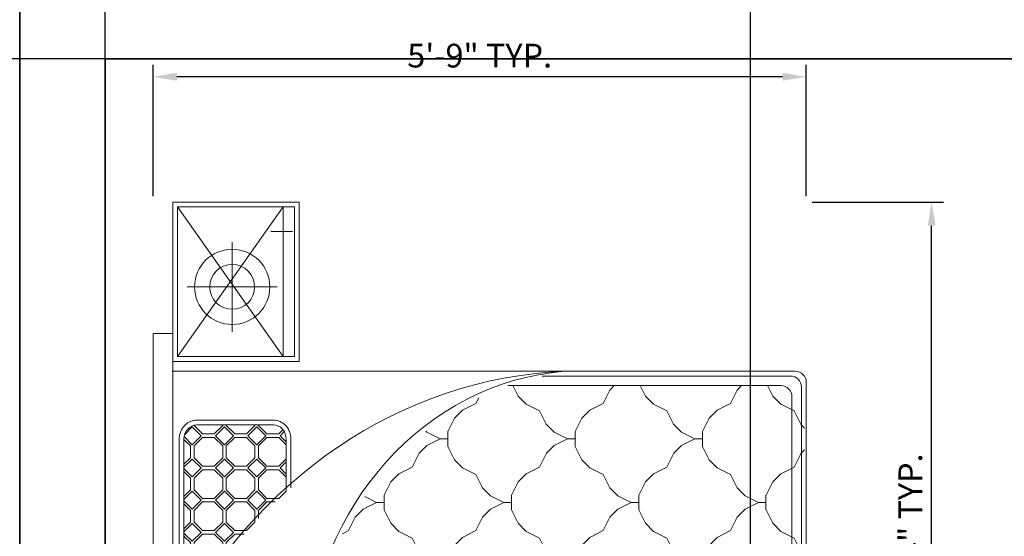
# Model space of a CAD drawing. Units: inches. Extents: x 1624 to 3956, y 1589 to 5028.
# Tile 13 of 16: x 1943 to 2046, y 2372 to 2426. Entities that reach past the tile are written whole.
import ezdxf

# ---------------------------------------------------------------- set-up
doc = ezdxf.new("R2010")
doc.units = ezdxf.units.IN
for name, color, linetype, lineweight in [('A-ANNO-DIMS', 2, 'Continuous', 13), ('A-FURN', 8, 'Continuous', 18), ('A-WALL', 7, 'Continuous', 35)]:
    doc.layers.add(name, color=color, linetype=linetype, lineweight=lineweight)
doc.styles.get("Standard").update_dxf_attribs({"font": 'arial.ttf'})
doc.dimstyles.new('Copy of ISO-25', dxfattribs={"dimtxt": 2.5, "dimasz": 2.5, "dimexe": 1.25, "dimexo": 0.625, "dimtad": 1, "dimdec": 1, "dimlunit": 4, "dimtxsty": 'Standard', "dimcen": 2.5, "dimadec": 0, "dimazin": 0, "dimtfac": 1, "dimtdec": 1, "dimtmove": 0, "dimatfit": 3, "dimfxl": 1, "dimarcsym": 0})

# ---------------------------------------------------------------- blocks, each defined once
blk = doc.blocks.new('A$C029D5C69')
for p, q in [((0.4164, 2.0693), (0.4164, 2.0066)), ((2.2315, 2.0693), (0.4164, 2.0693)), ((2.2315, 2.0066), (2.2315, 2.0693)), ((0, 1.606), (0, 2.0066)), ((0, 2.0066), (0.505, 2.0066)), ((0.4164, 2.0066), (2.2315, 2.0066)), ((0.505, 2.0066), (0.505, 1.606)), ((0.5252, 0.0351), (0.5252, 2.0066)), ((0.5403, 0.0502), (0.5403, 2.0066)), ((0.5706, 0.0805), (0.5706, 2.0066)), ((0.6869, 1.966), (0.6666, 2.0066)), ((0.7072, 2.0066), (0.6869, 1.966)), ((1.0902, 1.966), (1.0699, 2.0066)), ((1.1106, 2.0066), (1.0902, 1.966)), ((2.1114, 2.0087), (2.1114, 0.0351)), ((2.6479, 2.0066), (2.1429, 2.0066)), ((2.1429, 2.0066), (2.1429, 1.606)), ((2.6479, 1.606), (2.6479, 2.0066)), ((0.0151, 1.6211), (0.0151, 1.9915)), ((0.0151, 1.9915), (0.4899, 1.9915)), ((0.4899, 1.9915), (0.4899, 1.6211)), ((0.6869, 1.9425), (0.6869, 1.966)), ((0.6869, 1.9425), (0.6869, 1.966)), ((1.0902, 1.9425), (1.0902, 1.966)), ((1.0902, 1.9425), (1.0902, 1.966)), ((1.8954, 1.9865), (1.3081, 1.9865)), ((1.8954, 1.9713), (1.3339, 1.9713)), ((1.3849, 1.9713), (1.3656, 1.952)), ((1.3945, 1.9713), (1.3714, 1.9483)), ((1.4249, 1.945), (1.3986, 1.9713)), ((1.4288, 1.9507), (1.4081, 1.9713)), ((1.487, 1.9713), (1.4664, 1.9507)), ((1.4966, 1.9713), (1.4703, 1.945)), ((1.527, 1.945), (1.5007, 1.9713)), ((1.5309, 1.9507), (1.5102, 1.9713)), ((1.5891, 1.9713), (1.5685, 1.9507)), ((1.5987, 1.9713), (1.5724, 1.945)), ((1.6291, 1.945), (1.6028, 1.9713)), ((1.633, 1.9507), (1.6123, 1.9713)), ((1.6912, 1.9713), (1.6706, 1.9507)), ((1.7008, 1.9713), (1.6745, 1.945)), ((1.7312, 1.945), (1.7049, 1.9713)), ((1.7351, 1.9507), (1.7144, 1.9713)), ((1.7933, 1.9713), (1.7727, 1.9507)), ((1.8029, 1.9713), (1.7766, 1.945)), ((1.8333, 1.945), (1.807, 1.9713)), ((1.8372, 1.9507), (1.8165, 1.9713)), ((1.8954, 1.9713), (1.8748, 1.9507)), ((1.9043, 1.9707), (1.8787, 1.945)), ((1.9354, 1.945), (1.9114, 1.969)), ((2.6328, 1.9915), (2.158, 1.9915)), ((2.158, 1.9915), (2.158, 1.6211)), ((2.6328, 1.6211), (2.6328, 1.9915)), ((0.2689, 1.9609), (0.2689, 1.6764)), ((0.6634, 1.9425), (0.621, 1.9213)), ((0.6634, 1.9425), (0.621, 1.9213)), ((0.6869, 1.9425), (0.6634, 1.9425)), ((0.6869, 1.9425), (0.7104, 1.9425)), ((0.7528, 1.9213), (0.7104, 1.9425)), ((0.7528, 1.9213), (0.7104, 1.9425)), ((1.0668, 1.9425), (1.0244, 1.9213)), ((1.0668, 1.9425), (1.0244, 1.9213)), ((1.0902, 1.9425), (1.0668, 1.9425)), ((1.0902, 1.9425), (1.1137, 1.9425)), ((1.1561, 1.9213), (1.1137, 1.9425)), ((1.1561, 1.9213), (1.1137, 1.9425)), ((1.4249, 1.945), (1.4059, 1.926)), ((1.4288, 1.9394), (1.4116, 1.9222)), ((1.4476, 1.9507), (1.4288, 1.9507)), ((1.4288, 1.9393), (1.4476, 1.9393)), ((1.4476, 1.9507), (1.4664, 1.9507)), ((1.4664, 1.9393), (1.4476, 1.9393)), ((1.493, 1.9128), (1.4664, 1.9394)), ((1.4986, 1.9167), (1.4703, 1.945)), ((1.527, 1.945), (1.4986, 1.9167)), ((1.5309, 1.9394), (1.5043, 1.9128)), ((1.5497, 1.9507), (1.5309, 1.9507)), ((1.5309, 1.9393), (1.5497, 1.9393)), ((1.5497, 1.9507), (1.5685, 1.9507)), ((1.5685, 1.9393), (1.5497, 1.9393)), ((1.595, 1.9128), (1.5685, 1.9394)), ((1.6007, 1.9167), (1.5724, 1.945)), ((1.6291, 1.945), (1.6007, 1.9167)), ((1.633, 1.9394), (1.6064, 1.9128)), ((1.6518, 1.9507), (1.633, 1.9507)), ((1.633, 1.9393), (1.6518, 1.9393)), ((1.6518, 1.9507), (1.6706, 1.9507)), ((1.6706, 1.9393), (1.6518, 1.9393)), ((1.6971, 1.9128), (1.6706, 1.9394)), ((1.7028, 1.9167), (1.6745, 1.945)), ((1.7312, 1.945), (1.7028, 1.9167)), ((1.7351, 1.9394), (1.7085, 1.9128)), ((1.7539, 1.9507), (1.7351, 1.9507)), ((1.7351, 1.9393), (1.7539, 1.9393)), ((1.7539, 1.9507), (1.7727, 1.9507)), ((1.7727, 1.9393), (1.7539, 1.9393)), ((1.7992, 1.9128), (1.7727, 1.9394)), ((1.8049, 1.9167), (1.7766, 1.945)), ((1.8333, 1.945), (1.8049, 1.9167)), ((1.8372, 1.9394), (1.8106, 1.9128)), ((1.856, 1.9507), (1.8372, 1.9507)), ((1.8372, 1.9393), (1.856, 1.9393)), ((1.856, 1.9507), (1.8748, 1.9507)), ((1.8748, 1.9393), (1.856, 1.9393)), ((1.9013, 1.9128), (1.8748, 1.9394)), ((1.907, 1.9167), (1.8787, 1.945)), ((1.9354, 1.945), (1.907, 1.9167)), ((1.9393, 1.9394), (1.9127, 1.9128)), ((1.9393, 1.9393), (1.9404, 1.9393)), ((2.379, 1.9609), (2.379, 1.6764)), ((0.621, 1.9213), (0.5955, 1.8958)), ((0.7783, 1.8958), (0.7528, 1.9213)), ((1.0243, 1.9213), (0.9988, 1.8958)), ((1.1816, 1.8958), (1.1561, 1.9213)), ((1.493, 1.8752), (1.493, 1.9128)), ((1.5043, 1.8752), (1.5043, 1.9128)), ((1.595, 1.8752), (1.595, 1.9128)), ((1.6064, 1.8752), (1.6064, 1.9128)), ((1.6971, 1.8752), (1.6971, 1.9128)), ((1.7085, 1.8752), (1.7085, 1.9128)), ((1.7992, 1.8752), (1.7992, 1.9128)), ((1.8106, 1.8752), (1.8106, 1.9128)), ((1.9013, 1.8752), (1.9013, 1.9128)), ((1.9127, 1.8752), (1.9127, 1.9128)), ((1.9414, 1.688), (1.9414, 1.931)), ((1.9565, 1.688), (1.9565, 1.931)), ((0.5955, 1.8958), (0.5743, 1.8534)), ((0.7995, 1.8534), (0.7783, 1.8958)), ((0.9989, 1.8958), (0.9777, 1.8534)), ((1.2028, 1.8534), (1.1816, 1.8958)), ((1.493, 1.8752), (1.4867, 1.869)), ((1.5309, 1.8486), (1.5043, 1.8752)), ((1.595, 1.8752), (1.5685, 1.8486)), ((1.633, 1.8486), (1.6064, 1.8752)), ((1.6971, 1.8752), (1.6706, 1.8486)), ((1.7351, 1.8486), (1.7085, 1.8752)), ((1.7992, 1.8752), (1.7727, 1.8486)), ((1.8372, 1.8486), (1.8106, 1.8752)), ((1.9013, 1.8752), (1.8748, 1.8486)), ((1.9393, 1.8486), (1.9127, 1.8752)), ((0.5743, 1.8534), (0.5706, 1.8515)), ((0.5743, 1.8534), (0.5706, 1.8515)), ((0.8419, 1.8322), (0.7995, 1.8534)), ((0.8419, 1.8322), (0.7995, 1.8534)), ((0.9777, 1.8534), (0.9353, 1.8322)), ((0.9777, 1.8534), (0.9353, 1.8322)), ((1.2452, 1.8322), (1.2028, 1.8534)), ((1.2452, 1.8322), (1.2028, 1.8534)), ((1.4986, 1.8713), (1.4922, 1.8648)), ((1.527, 1.8429), (1.4986, 1.8713)), ((1.527, 1.8429), (1.5242, 1.8401)), ((1.5497, 1.8486), (1.5309, 1.8486)), ((1.5497, 1.8486), (1.5685, 1.8486)), ((1.6007, 1.8713), (1.5724, 1.8429)), ((1.6007, 1.8146), (1.5724, 1.8429)), ((1.6291, 1.8429), (1.6007, 1.8713)), ((1.6291, 1.8429), (1.6007, 1.8146)), ((1.6518, 1.8486), (1.633, 1.8486)), ((1.6518, 1.8486), (1.6706, 1.8486)), ((1.7028, 1.8713), (1.6745, 1.8429)), ((1.7028, 1.8146), (1.6745, 1.8429)), ((1.7312, 1.8429), (1.7028, 1.8713)), ((1.7312, 1.8429), (1.7028, 1.8146)), ((1.7539, 1.8486), (1.7351, 1.8486)), ((1.7539, 1.8486), (1.7727, 1.8486)), ((1.8049, 1.8713), (1.7766, 1.8429)), ((1.8049, 1.8146), (1.7766, 1.8429)), ((1.8333, 1.8429), (1.8049, 1.8713)), ((1.8333, 1.8429), (1.8049, 1.8146)), ((1.856, 1.8486), (1.8372, 1.8486)), ((1.856, 1.8486), (1.8748, 1.8486)), ((1.907, 1.8713), (1.8787, 1.8429)), ((1.907, 1.8146), (1.8787, 1.8429)), ((1.9354, 1.8429), (1.907, 1.8713)), ((1.9354, 1.8429), (1.907, 1.8146)), ((1.9414, 1.8486), (1.9393, 1.8486)), ((0.1267, 1.8186), (0.4111, 1.8186)), ((0.8674, 1.8067), (0.8419, 1.8322)), ((0.9352, 1.8322), (0.9097, 1.8067)), ((1.2707, 1.8067), (1.2452, 1.8322)), ((1.5309, 1.8373), (1.5295, 1.8359)), ((1.5309, 1.8373), (1.5497, 1.8373)), ((1.5685, 1.8373), (1.5497, 1.8373)), ((1.595, 1.8107), (1.5685, 1.8373)), ((1.595, 1.7806), (1.595, 1.8107)), ((1.633, 1.8373), (1.6064, 1.8107)), ((1.6064, 1.7731), (1.6064, 1.8107)), ((1.633, 1.8373), (1.6518, 1.8373)), ((1.6706, 1.8373), (1.6518, 1.8373)), ((1.6971, 1.8107), (1.6706, 1.8373)), ((1.6971, 1.7731), (1.6971, 1.8107)), ((1.7351, 1.8373), (1.7085, 1.8107)), ((1.7085, 1.7731), (1.7085, 1.8107)), ((1.7351, 1.8373), (1.7539, 1.8373)), ((1.7727, 1.8373), (1.7539, 1.8373)), ((1.7992, 1.8107), (1.7727, 1.8373)), ((1.7992, 1.7731), (1.7992, 1.8107)), ((1.8372, 1.8373), (1.8106, 1.8107)), ((1.8106, 1.7731), (1.8106, 1.8107)), ((1.8372, 1.8373), (1.856, 1.8373)), ((1.8748, 1.8373), (1.856, 1.8373)), ((1.9013, 1.8107), (1.8748, 1.8373)), ((1.9013, 1.7731), (1.9013, 1.8107)), ((1.9393, 1.8373), (1.9127, 1.8107)), ((1.9127, 1.7731), (1.9127, 1.8107)), ((1.9393, 1.8373), (1.9414, 1.8373)), ((2.2367, 1.8186), (2.5212, 1.8186)), ((0.8886, 1.7643), (0.8674, 1.8067)), ((0.9098, 1.8067), (0.8886, 1.7643)), ((1.2919, 1.7643), (1.2707, 1.8067)), ((0.8886, 1.7408), (0.8886, 1.7643)), ((1.2981, 1.7768), (1.2919, 1.7643)), ((1.2919, 1.7519), (1.2919, 1.7643)), ((1.633, 1.7465), (1.6064, 1.7731)), ((1.6971, 1.7731), (1.6706, 1.7465)), ((1.7028, 1.7692), (1.6745, 1.7408)), ((1.7312, 1.7408), (1.7028, 1.7692)), ((1.7351, 1.7465), (1.7085, 1.7731)), ((1.7992, 1.7731), (1.7727, 1.7465)), ((1.8049, 1.7692), (1.7766, 1.7408)), ((1.8333, 1.7408), (1.8049, 1.7692)), ((1.8372, 1.7465), (1.8106, 1.7731)), ((1.9013, 1.7731), (1.8748, 1.7465)), ((1.907, 1.7692), (1.8787, 1.7408)), ((1.9354, 1.7408), (1.907, 1.7692)), ((1.9393, 1.7465), (1.9127, 1.7731)), ((0.8227, 1.7196), (0.7972, 1.6941)), ((0.8651, 1.7408), (0.8227, 1.7196)), ((0.8651, 1.7408), (0.8227, 1.7196)), ((0.912, 1.7408), (0.8651, 1.7408)), ((0.9544, 1.7196), (0.912, 1.7408)), ((0.9544, 1.7196), (0.912, 1.7408)), ((0.98, 1.6941), (0.9545, 1.7196)), ((1.226, 1.7196), (1.2005, 1.6941)), ((1.2684, 1.7408), (1.226, 1.7196)), ((1.2684, 1.7408), (1.226, 1.7196)), ((1.2885, 1.7408), (1.2684, 1.7408)), ((1.6518, 1.7465), (1.633, 1.7465)), ((1.6443, 1.7352), (1.6518, 1.7352)), ((1.6518, 1.7465), (1.6706, 1.7465)), ((1.6706, 1.7352), (1.6518, 1.7352)), ((1.6971, 1.7086), (1.6706, 1.7352)), ((1.7028, 1.7125), (1.6745, 1.7408)), ((1.7312, 1.7408), (1.7028, 1.7125)), ((1.7351, 1.7352), (1.7085, 1.7086)), ((1.7539, 1.7465), (1.7351, 1.7465)), ((1.7351, 1.7352), (1.7539, 1.7352)), ((1.7539, 1.7465), (1.7727, 1.7465)), ((1.7727, 1.7352), (1.7539, 1.7352)), ((1.7992, 1.7086), (1.7727, 1.7352)), ((1.8049, 1.7125), (1.7766, 1.7408)), ((1.8333, 1.7408), (1.8049, 1.7125)), ((1.8372, 1.7352), (1.8106, 1.7086)), ((1.856, 1.7465), (1.8372, 1.7465)), ((1.8372, 1.7352), (1.856, 1.7352)), ((1.856, 1.7465), (1.8748, 1.7465)), ((1.8748, 1.7352), (1.856, 1.7352)), ((1.9013, 1.7086), (1.8748, 1.7352)), ((1.907, 1.7125), (1.8787, 1.7408)), ((1.9354, 1.7408), (1.907, 1.7125)), ((1.9393, 1.7352), (1.9127, 1.7086)), ((1.9414, 1.7465), (1.9393, 1.7465)), ((1.9393, 1.7352), (1.9414, 1.7352)), ((0.5766, 1.6941), (0.5706, 1.7002)), ((0.5978, 1.6517), (0.5766, 1.6941)), ((0.7972, 1.6941), (0.776, 1.6517)), ((1.0011, 1.6517), (0.9799, 1.6941)), ((1.2005, 1.6941), (1.1793, 1.6517)), ((1.6971, 1.682), (1.6971, 1.7086)), ((1.7085, 1.671), (1.7085, 1.7086)), ((1.7992, 1.671), (1.7992, 1.7086)), ((1.8106, 1.671), (1.8106, 1.7086)), ((1.9013, 1.671), (1.9013, 1.7086)), ((1.9127, 1.671), (1.9127, 1.7086)), ((2.5551, 1.6275), (2.5551, 1.696)), ((1.7318, 1.6477), (1.7085, 1.671)), ((1.7992, 1.671), (1.7759, 1.6477)), ((1.8049, 1.6671), (1.7855, 1.6477)), ((1.8244, 1.6477), (1.8049, 1.6671)), ((1.8339, 1.6477), (1.8106, 1.671)), ((1.9013, 1.671), (1.878, 1.6477)), ((1.907, 1.6671), (1.8876, 1.6477)), ((1.9202, 1.6539), (1.907, 1.6671)), ((1.926, 1.6577), (1.9127, 1.671)), ((0.6402, 1.6305), (0.5978, 1.6517)), ((0.6402, 1.6305), (0.5978, 1.6517)), ((0.6657, 1.605), (0.6402, 1.6305)), ((0.7336, 1.6305), (0.7081, 1.605)), ((0.776, 1.6517), (0.7336, 1.6305)), ((0.776, 1.6517), (0.7336, 1.6305)), ((1.0435, 1.6305), (1.0011, 1.6517)), ((1.0435, 1.6305), (1.0011, 1.6517)), ((1.0691, 1.605), (1.0436, 1.6305)), ((1.1369, 1.6305), (1.1114, 1.605)), ((1.1793, 1.6517), (1.1369, 1.6305)), ((1.1793, 1.6517), (1.1369, 1.6305)), ((1.8961, 1.6477), (1.7289, 1.6477)), ((1.8961, 1.6325), (1.7422, 1.6325)), ((0.505, 1.606), (0, 1.606)), ((0.4899, 1.6211), (0.0151, 1.6211)), ((0.6869, 1.5626), (0.6657, 1.605)), ((0.7081, 1.605), (0.6869, 1.5626)), ((1.0902, 1.5626), (1.069, 1.605)), ((1.1114, 1.605), (1.0902, 1.5626)), ((2.1429, 1.606), (2.6479, 1.606)), ((2.158, 1.6211), (2.6328, 1.6211)), ((0.6869, 1.5392), (0.6869, 1.5626)), ((0.6869, 1.5392), (0.6869, 1.5626)), ((1.0902, 1.5392), (1.0902, 1.5626)), ((1.0902, 1.5392), (1.0902, 1.5626)), ((0.6634, 1.5391), (0.621, 1.5179)), ((0.6634, 1.5391), (0.621, 1.5179)), ((0.6869, 1.5392), (0.6634, 1.5392)), ((0.6869, 1.5392), (0.7104, 1.5392)), ((0.7528, 1.5179), (0.7104, 1.5391)), ((0.7528, 1.5179), (0.7104, 1.5391)), ((1.0668, 1.5391), (1.0244, 1.5179)), ((1.0668, 1.5391), (1.0244, 1.5179)), ((1.0902, 1.5392), (1.0668, 1.5392)), ((1.0902, 1.5392), (1.1137, 1.5392)), ((1.1561, 1.5179), (1.1137, 1.5391)), ((1.1561, 1.5179), (1.1137, 1.5391)), ((1.4534, 1.5308), (1.4277, 1.5179)), ((1.4534, 1.5308), (1.4277, 1.5179)), ((0.621, 1.5179), (0.5955, 1.4924)), ((0.7783, 1.4924), (0.7528, 1.5179)), ((1.0243, 1.5179), (0.9988, 1.4924)), ((1.1816, 1.4924), (1.1561, 1.5179)), ((1.4277, 1.5179), (1.4022, 1.4924)), ((0.5955, 1.4925), (0.5743, 1.4501)), ((0.7995, 1.4501), (0.7783, 1.4925)), ((0.9989, 1.4925), (0.9777, 1.4501)), ((1.2028, 1.4501), (1.1816, 1.4925)), ((1.4022, 1.4925), (1.381, 1.4501)), ((1.6062, 1.4501), (1.5966, 1.4692)), ((0.5743, 1.45), (0.5706, 1.4481)), ((0.5743, 1.45), (0.5706, 1.4481)), ((0.8419, 1.4288), (0.7995, 1.45)), ((0.8419, 1.4288), (0.7995, 1.45)), ((0.9777, 1.45), (0.9353, 1.4288)), ((0.9777, 1.45), (0.9353, 1.4288)), ((1.2452, 1.4288), (1.2028, 1.45)), ((1.2452, 1.4288), (1.2028, 1.45)), ((1.381, 1.45), (1.3386, 1.4288)), ((1.381, 1.45), (1.3386, 1.4288)), ((1.6486, 1.4288), (1.6062, 1.45)), ((1.6486, 1.4288), (1.6062, 1.45)), ((0.5403, 1.4117), (0.5706, 1.4117)), ((0.8674, 1.4033), (0.8419, 1.4288)), ((0.9352, 1.4288), (0.9097, 1.4033)), ((1.2707, 1.4033), (1.2452, 1.4288)), ((1.3386, 1.4288), (1.3131, 1.4033)), ((1.6741, 1.4033), (1.6486, 1.4288)), ((0.8886, 1.361), (0.8674, 1.4034)), ((0.9098, 1.4034), (0.8886, 1.361)), ((1.2919, 1.361), (1.2707, 1.4034)), ((1.3131, 1.4034), (1.2919, 1.361)), ((1.6953, 1.361), (1.6741, 1.4034)), ((1.714, 1.3984), (1.6953, 1.361)), ((0.8886, 1.3375), (0.8886, 1.3609)), ((1.2919, 1.3375), (1.2919, 1.3609)), ((1.6953, 1.3375), (1.6953, 1.3609)), ((0.8227, 1.3163), (0.7972, 1.2908)), ((0.8651, 1.3374), (0.8227, 1.3162)), ((0.8651, 1.3374), (0.8227, 1.3162)), ((0.912, 1.3375), (0.8651, 1.3375)), ((0.9544, 1.3162), (0.912, 1.3374)), ((0.9544, 1.3162), (0.912, 1.3374)), ((0.98, 1.2908), (0.9545, 1.3163)), ((1.226, 1.3163), (1.2005, 1.2908)), ((1.2684, 1.3374), (1.226, 1.3162)), ((1.2684, 1.3374), (1.226, 1.3162)), ((1.3154, 1.3375), (1.2684, 1.3375)), ((1.3578, 1.3162), (1.3154, 1.3374)), ((1.3578, 1.3162), (1.3154, 1.3374)), ((1.3833, 1.2908), (1.3578, 1.3163)), ((1.6294, 1.3163), (1.6039, 1.2908)), ((1.6718, 1.3374), (1.6294, 1.3162)), ((1.6718, 1.3374), (1.6294, 1.3162)), ((1.7187, 1.3375), (1.6718, 1.3375)), ((1.7611, 1.3162), (1.7187, 1.3374)), ((1.7611, 1.3162), (1.7187, 1.3374)), ((1.7867, 1.2908), (1.7611, 1.3163)), ((0.5766, 1.2908), (0.5706, 1.2968)), ((0.5978, 1.2484), (0.5766, 1.2908)), ((0.7972, 1.2908), (0.776, 1.2484)), ((1.0011, 1.2484), (0.9799, 1.2908)), ((1.2005, 1.2908), (1.1793, 1.2484)), ((1.4045, 1.2484), (1.3833, 1.2908)), ((1.6039, 1.2908), (1.5827, 1.2484)), ((1.8078, 1.2484), (1.7866, 1.2908)), ((0.6402, 1.2271), (0.5978, 1.2483)), ((0.6402, 1.2271), (0.5978, 1.2483)), ((0.776, 1.2483), (0.7336, 1.2271)), ((0.776, 1.2483), (0.7336, 1.2271)), ((1.0435, 1.2271), (1.0011, 1.2483)), ((1.0435, 1.2271), (1.0011, 1.2483)), ((1.1793, 1.2483), (1.1369, 1.2271)), ((1.1793, 1.2483), (1.1369, 1.2271)), ((1.4469, 1.2271), (1.4045, 1.2483)), ((1.4469, 1.2271), (1.4045, 1.2483)), ((1.5827, 1.2483), (1.5403, 1.2271)), ((1.5827, 1.2483), (1.5403, 1.2271)), ((1.8502, 1.2271), (1.8078, 1.2483)), ((1.8502, 1.2271), (1.8078, 1.2483)), ((0.6657, 1.2017), (0.6402, 1.2272)), ((0.7336, 1.2272), (0.7081, 1.2017)), ((1.0691, 1.2017), (1.0436, 1.2272)), ((1.1369, 1.2272), (1.1114, 1.2017)), ((1.4724, 1.2017), (1.4469, 1.2272)), ((1.5403, 1.2272), (1.5148, 1.2017)), ((1.8758, 1.2017), (1.8503, 1.2272)), ((0.5403, 1.21), (0.5706, 1.21)), ((0.6869, 1.1593), (0.6657, 1.2017)), ((0.7081, 1.2017), (0.6869, 1.1593)), ((1.0902, 1.1593), (1.069, 1.2017)), ((1.1114, 1.2017), (1.0902, 1.1593)), ((1.4936, 1.1593), (1.4724, 1.2017)), ((1.5148, 1.2017), (1.4936, 1.1593)), ((1.8969, 1.1593), (1.8757, 1.2017)), ((1.9181, 1.2017), (1.8969, 1.1593)), ((1.9215, 1.2051), (1.9181, 1.2017)), ((0.6869, 1.1358), (0.6869, 1.1593)), ((0.6869, 1.1358), (0.6869, 1.1593)), ((1.0902, 1.1358), (1.0902, 1.1593)), ((1.0902, 1.1358), (1.0902, 1.1593)), ((1.4936, 1.1358), (1.4936, 1.1593)), ((1.4936, 1.1358), (1.4936, 1.1593)), ((1.8969, 1.1358), (1.8969, 1.1593)), ((1.8969, 1.1358), (1.8969, 1.1593)), ((0.6634, 1.1358), (0.621, 1.1146)), ((0.6634, 1.1358), (0.621, 1.1146)), ((0.6869, 1.1358), (0.6634, 1.1358)), ((0.6869, 1.1358), (0.7104, 1.1358)), ((0.7528, 1.1146), (0.7104, 1.1358)), ((0.7528, 1.1146), (0.7104, 1.1358)), ((1.0668, 1.1358), (1.0244, 1.1146)), ((1.0668, 1.1358), (1.0244, 1.1146)), ((1.0902, 1.1358), (1.0668, 1.1358)), ((1.0902, 1.1358), (1.1137, 1.1358)), ((1.1561, 1.1146), (1.1137, 1.1358)), ((1.1561, 1.1146), (1.1137, 1.1358)), ((1.4701, 1.1358), (1.4277, 1.1146)), ((1.4701, 1.1358), (1.4277, 1.1146)), ((1.4936, 1.1358), (1.4701, 1.1358)), ((1.4936, 1.1358), (1.5171, 1.1358)), ((1.5595, 1.1146), (1.5171, 1.1358)), ((1.5595, 1.1146), (1.5171, 1.1358)), ((1.8735, 1.1358), (1.8311, 1.1146)), ((1.8735, 1.1358), (1.8311, 1.1146)), ((1.8969, 1.1358), (1.8735, 1.1358)), ((1.8969, 1.1358), (1.9204, 1.1358)), ((1.9628, 1.1146), (1.9204, 1.1358)), ((1.9628, 1.1146), (1.9204, 1.1358)), ((0.621, 1.1146), (0.5955, 1.0891)), ((0.7783, 1.0891), (0.7528, 1.1146)), ((1.0243, 1.1146), (0.9988, 1.0891)), ((1.1816, 1.0891), (1.1561, 1.1146)), ((1.4277, 1.1146), (1.4022, 1.0891)), ((1.585, 1.0891), (1.5595, 1.1146)), ((1.831, 1.1146), (1.8055, 1.0891)), ((1.9883, 1.0891), (1.9628, 1.1146)), ((0.5955, 1.0891), (0.5743, 1.0467)), ((0.7995, 1.0467), (0.7783, 1.0891)), ((0.9989, 1.0891), (0.9777, 1.0467)), ((1.2028, 1.0467), (1.1816, 1.0891)), ((1.4022, 1.0891), (1.381, 1.0467)), ((1.6062, 1.0467), (1.585, 1.0891)), ((1.8056, 1.0891), (1.7844, 1.0467)), ((2.0095, 1.0467), (1.9883, 1.0891)), ((0.5743, 1.0467), (0.5706, 1.0448)), ((0.5743, 1.0467), (0.5706, 1.0448)), ((0.8419, 1.0255), (0.7995, 1.0467)), ((0.8419, 1.0255), (0.7995, 1.0467)), ((0.9777, 1.0467), (0.9353, 1.0255)), ((0.9777, 1.0467), (0.9353, 1.0255)), ((1.2452, 1.0255), (1.2028, 1.0467)), ((1.2452, 1.0255), (1.2028, 1.0467)), ((1.381, 1.0467), (1.3386, 1.0255)), ((1.381, 1.0467), (1.3386, 1.0255)), ((1.6486, 1.0255), (1.6062, 1.0467)), ((1.6486, 1.0255), (1.6062, 1.0467)), ((1.7844, 1.0467), (1.742, 1.0255)), ((1.7844, 1.0467), (1.742, 1.0255)), ((2.0276, 1.0376), (2.0095, 1.0467)), ((2.0276, 1.0376), (2.0095, 1.0467)), ((0.8674, 1), (0.8419, 1.0255)), ((0.8886, 0.9576), (0.8674, 1)), ((0.9098, 1), (0.8886, 0.9576)), ((0.9352, 1.0255), (0.9097, 1)), ((1.2707, 1), (1.2452, 1.0255)), ((1.2919, 0.9576), (1.2707, 1)), ((1.3131, 1), (1.2919, 0.9576)), ((1.3386, 1.0255), (1.3131, 1)), ((1.6741, 1), (1.6486, 1.0255)), ((1.6953, 0.9576), (1.6741, 1)), ((1.7165, 1), (1.6953, 0.9576)), ((1.7419, 1.0255), (1.7164, 1)), ((0.8886, 0.9341), (0.8886, 0.9576)), ((1.2919, 0.9341), (1.2919, 0.9576)), ((1.6953, 0.9341), (1.6953, 0.9576)), ((2.066, 0.9457), (2.066, 0.0805)), ((0.8227, 0.9129), (0.7972, 0.8874)), ((0.8651, 0.9341), (0.8227, 0.9129)), ((0.8651, 0.9341), (0.8227, 0.9129)), ((0.912, 0.9341), (0.8651, 0.9341)), ((0.9544, 0.9129), (0.912, 0.9341)), ((0.9544, 0.9129), (0.912, 0.9341)), ((0.98, 0.8874), (0.9545, 0.9129)), ((1.226, 0.9129), (1.2005, 0.8874)), ((1.2684, 0.9341), (1.226, 0.9129)), ((1.2684, 0.9341), (1.226, 0.9129)), ((1.3154, 0.9341), (1.2684, 0.9341)), ((1.3578, 0.9129), (1.3154, 0.9341)), ((1.3578, 0.9129), (1.3154, 0.9341)), ((1.3833, 0.8874), (1.3578, 0.9129)), ((1.6294, 0.9129), (1.6039, 0.8874)), ((1.6718, 0.9341), (1.6294, 0.9129)), ((1.6718, 0.9341), (1.6294, 0.9129)), ((1.7187, 0.9341), (1.6718, 0.9341)), ((1.7611, 0.9129), (1.7187, 0.9341)), ((1.7611, 0.9129), (1.7187, 0.9341)), ((1.7867, 0.8874), (1.7611, 0.9129)), ((2.0327, 0.9129), (2.0072, 0.8874)), ((2.066, 0.9295), (2.0327, 0.9129)), ((2.066, 0.9295), (2.0327, 0.9129)), ((0.5766, 0.8874), (0.5706, 0.8935)), ((0.5978, 0.845), (0.5766, 0.8874)), ((0.7972, 0.8874), (0.776, 0.845)), ((1.0011, 0.845), (0.9799, 0.8874)), ((1.2005, 0.8874), (1.1793, 0.845)), ((1.4045, 0.845), (1.3833, 0.8874)), ((1.6039, 0.8874), (1.5827, 0.845)), ((1.8078, 0.845), (1.7866, 0.8874)), ((2.0072, 0.8874), (1.986, 0.845)), ((0.6402, 0.8238), (0.5978, 0.845)), ((0.6402, 0.8238), (0.5978, 0.845)), ((0.776, 0.845), (0.7336, 0.8238)), ((0.776, 0.845), (0.7336, 0.8238)), ((1.0435, 0.8238), (1.0011, 0.845)), ((1.0435, 0.8238), (1.0011, 0.845)), ((1.1793, 0.845), (1.1369, 0.8238)), ((1.1793, 0.845), (1.1369, 0.8238)), ((1.4469, 0.8238), (1.4045, 0.845)), ((1.4469, 0.8238), (1.4045, 0.845)), ((1.5827, 0.845), (1.5403, 0.8238)), ((1.5827, 0.845), (1.5403, 0.8238)), ((1.8502, 0.8238), (1.8078, 0.845)), ((1.8502, 0.8238), (1.8078, 0.845)), ((1.986, 0.845), (1.9436, 0.8238)), ((1.986, 0.845), (1.9436, 0.8238)), ((0.6657, 0.7983), (0.6402, 0.8238)), ((0.7336, 0.8238), (0.7081, 0.7983)), ((1.0691, 0.7983), (1.0436, 0.8238)), ((1.1369, 0.8238), (1.1114, 0.7983)), ((1.4724, 0.7983), (1.4469, 0.8238)), ((1.5403, 0.8238), (1.5148, 0.7983)), ((1.8758, 0.7983), (1.8503, 0.8238)), ((1.9436, 0.8238), (1.9181, 0.7983)), ((2.0962, 0.8369), (2.0962, 0.0502)), ((0.6869, 0.7559), (0.6657, 0.7983)), ((0.7081, 0.7983), (0.6869, 0.7559)), ((1.0902, 0.7559), (1.069, 0.7983)), ((1.1114, 0.7983), (1.0902, 0.7559)), ((1.4936, 0.7559), (1.4724, 0.7983)), ((1.5148, 0.7983), (1.4936, 0.7559)), ((1.8969, 0.7559), (1.8757, 0.7983)), ((1.9181, 0.7983), (1.8969, 0.7559)), ((0.6869, 0.7325), (0.6869, 0.7559)), ((0.6869, 0.7325), (0.6869, 0.7559)), ((1.0902, 0.7325), (1.0902, 0.7559)), ((1.0902, 0.7325), (1.0902, 0.7559)), ((1.2024, 0.7028), (1.2503, 0.7507)), ((1.4936, 0.7325), (1.4936, 0.7559)), ((1.4936, 0.7325), (1.4936, 0.7559)), ((1.8969, 0.7325), (1.8969, 0.7559)), ((1.8969, 0.7325), (1.8969, 0.7559)), ((0.6634, 0.7324), (0.621, 0.7112)), ((0.6634, 0.7324), (0.621, 0.7112)), ((0.6869, 0.7325), (0.6634, 0.7325)), ((0.6869, 0.7325), (0.7104, 0.7325)), ((0.7528, 0.7112), (0.7104, 0.7324)), ((0.7528, 0.7112), (0.7104, 0.7324)), ((1.0668, 0.7324), (1.0244, 0.7112)), ((1.0668, 0.7324), (1.0244, 0.7112)), ((1.0902, 0.7325), (1.0668, 0.7325)), ((1.0902, 0.7325), (1.1137, 0.7325)), ((1.1561, 0.7112), (1.1137, 0.7324)), ((1.1561, 0.7112), (1.1137, 0.7324)), ((1.4701, 0.7324), (1.4277, 0.7112)), ((1.4701, 0.7324), (1.4277, 0.7112)), ((1.4936, 0.7325), (1.4701, 0.7325)), ((1.4936, 0.7325), (1.5171, 0.7325)), ((1.5595, 0.7112), (1.5171, 0.7324)), ((1.5595, 0.7112), (1.5171, 0.7324)), ((1.8735, 0.7324), (1.8311, 0.7112)), ((1.8735, 0.7324), (1.8311, 0.7112)), ((1.8969, 0.7325), (1.8735, 0.7325)), ((1.8969, 0.7325), (1.9204, 0.7325)), ((1.9628, 0.7112), (1.9204, 0.7324)), ((1.9628, 0.7112), (1.9204, 0.7324)), ((0.621, 0.7113), (0.5955, 0.6858)), ((0.7783, 0.6858), (0.7528, 0.7113)), ((1.0243, 0.7113), (0.9988, 0.6858)), ((1.1816, 0.6858), (1.1561, 0.7113)), ((1.4277, 0.7113), (1.4022, 0.6858)), ((1.585, 0.6858), (1.5595, 0.7113)), ((1.831, 0.7113), (1.8055, 0.6858)), ((1.9883, 0.6858), (1.9628, 0.7113)), ((0.5955, 0.6858), (0.5743, 0.6434)), ((0.7995, 0.6434), (0.7783, 0.6858)), ((0.9989, 0.6858), (0.9777, 0.6434)), ((1.2028, 0.6434), (1.1816, 0.6858)), ((1.4022, 0.6858), (1.381, 0.6434)), ((1.6062, 0.6434), (1.585, 0.6858)), ((1.8056, 0.6858), (1.7844, 0.6434)), ((2.0095, 0.6434), (1.9883, 0.6858)), ((0.5743, 0.6433), (0.5706, 0.6414)), ((0.5743, 0.6433), (0.5706, 0.6414)), ((0.8419, 0.6221), (0.7995, 0.6433)), ((0.8419, 0.6221), (0.7995, 0.6433)), ((0.9777, 0.6433), (0.9353, 0.6221)), ((0.9777, 0.6433), (0.9353, 0.6221)), ((1.2452, 0.6221), (1.2028, 0.6433)), ((1.2452, 0.6221), (1.2028, 0.6433)), ((1.381, 0.6433), (1.3386, 0.6221)), ((1.381, 0.6433), (1.3386, 0.6221)), ((1.6486, 0.6221), (1.6062, 0.6433)), ((1.6486, 0.6221), (1.6062, 0.6433)), ((1.7844, 0.6433), (1.742, 0.6221)), ((1.7844, 0.6433), (1.742, 0.6221)), ((2.0519, 0.6221), (2.0095, 0.6433)), ((2.0519, 0.6221), (2.0095, 0.6433)), ((0.8674, 0.5967), (0.8419, 0.6222)), ((0.8886, 0.5543), (0.8674, 0.5967)), ((0.9098, 0.5967), (0.8886, 0.5543)), ((0.9352, 0.6222), (0.9097, 0.5967)), ((1.2707, 0.5967), (1.2452, 0.6222)), ((1.2919, 0.5543), (1.2707, 0.5967)), ((1.3131, 0.5967), (1.2919, 0.5543)), ((1.3386, 0.6222), (1.3131, 0.5967)), ((1.6741, 0.5967), (1.6486, 0.6222)), ((1.6953, 0.5543), (1.6741, 0.5967)), ((1.7165, 0.5967), (1.6953, 0.5543)), ((1.7419, 0.6222), (1.7164, 0.5967)), ((2.066, 0.6081), (2.0519, 0.6222)), ((0.8651, 0.5308), (0.8227, 0.5096)), ((0.8651, 0.5308), (0.8227, 0.5096)), ((0.912, 0.5308), (0.8651, 0.5308)), ((0.8886, 0.5308), (0.8886, 0.5543)), ((0.9544, 0.5096), (0.912, 0.5308)), ((0.9544, 0.5096), (0.912, 0.5308)), ((1.2684, 0.5308), (1.226, 0.5096)), ((1.2684, 0.5308), (1.226, 0.5096)), ((1.3154, 0.5308), (1.2684, 0.5308)), ((1.2919, 0.5308), (1.2919, 0.5543)), ((1.3578, 0.5096), (1.3154, 0.5308)), ((1.3578, 0.5096), (1.3154, 0.5308)), ((1.6718, 0.5308), (1.6294, 0.5096)), ((1.6718, 0.5308), (1.6294, 0.5096)), ((1.7187, 0.5308), (1.6718, 0.5308)), ((1.6953, 0.5308), (1.6953, 0.5543)), ((1.7611, 0.5096), (1.7187, 0.5308)), ((1.7611, 0.5096), (1.7187, 0.5308)), ((0.8227, 0.5096), (0.7972, 0.4841)), ((0.98, 0.4841), (0.9545, 0.5096)), ((1.226, 0.5096), (1.2005, 0.4841)), ((1.3833, 0.4841), (1.3578, 0.5096)), ((1.6294, 0.5096), (1.6039, 0.4841)), ((1.7867, 0.4841), (1.7611, 0.5096)), ((2.0327, 0.5096), (2.0072, 0.4841)), ((2.066, 0.5262), (2.0327, 0.5096)), ((2.066, 0.5262), (2.0327, 0.5096)), ((0.5766, 0.4841), (0.5706, 0.4901)), ((0.5978, 0.4417), (0.5766, 0.4841)), ((0.7972, 0.4841), (0.776, 0.4417)), ((1.0011, 0.4417), (0.9799, 0.4841)), ((1.2005, 0.4841), (1.1793, 0.4417)), ((1.4045, 0.4417), (1.3833, 0.4841)), ((1.6039, 0.4841), (1.5827, 0.4417)), ((1.8078, 0.4417), (1.7866, 0.4841)), ((2.0072, 0.4841), (1.986, 0.4417)), ((0.6402, 0.4205), (0.5978, 0.4417)), ((0.6402, 0.4205), (0.5978, 0.4417)), ((0.776, 0.4417), (0.7336, 0.4205)), ((0.776, 0.4417), (0.7336, 0.4205)), ((1.0435, 0.4205), (1.0011, 0.4417)), ((1.0435, 0.4205), (1.0011, 0.4417)), ((1.1793, 0.4417), (1.1369, 0.4205)), ((1.1793, 0.4417), (1.1369, 0.4205)), ((1.4469, 0.4205), (1.4045, 0.4417)), ((1.4469, 0.4205), (1.4045, 0.4417)), ((1.5827, 0.4417), (1.5403, 0.4205)), ((1.5827, 0.4417), (1.5403, 0.4205)), ((1.8502, 0.4205), (1.8078, 0.4417)), ((1.8502, 0.4205), (1.8078, 0.4417)), ((1.986, 0.4417), (1.9436, 0.4205)), ((1.986, 0.4417), (1.9436, 0.4205)), ((0.6657, 0.395), (0.6402, 0.4205)), ((0.7336, 0.4205), (0.7081, 0.395)), ((1.0691, 0.395), (1.0436, 0.4205)), ((1.1369, 0.4205), (1.1114, 0.395)), ((1.4724, 0.395), (1.4469, 0.4205)), ((1.5403, 0.4205), (1.5148, 0.395)), ((1.8758, 0.395), (1.8503, 0.4205)), ((1.9436, 0.4205), (1.9181, 0.395)), ((0.6869, 0.3526), (0.6657, 0.395)), ((0.7081, 0.395), (0.6869, 0.3526)), ((1.0902, 0.3526), (1.069, 0.395)), ((1.1114, 0.395), (1.0902, 0.3526)), ((1.4936, 0.3526), (1.4724, 0.395)), ((1.5148, 0.395), (1.4936, 0.3526)), ((1.8969, 0.3526), (1.8757, 0.395)), ((1.9181, 0.395), (1.8969, 0.3526)), ((0.6869, 0.3291), (0.6869, 0.3526)), ((0.6869, 0.3291), (0.6869, 0.3526)), ((1.0902, 0.3291), (1.0902, 0.3526)), ((1.0902, 0.3291), (1.0902, 0.3526)), ((1.4936, 0.3291), (1.4936, 0.3526)), ((1.4936, 0.3291), (1.4936, 0.3526)), ((1.8969, 0.3291), (1.8969, 0.3526)), ((1.8969, 0.3291), (1.8969, 0.3526)), ((0.6634, 0.3291), (0.621, 0.3079)), ((0.6634, 0.3291), (0.621, 0.3079)), ((0.6869, 0.3291), (0.6634, 0.3291)), ((0.6869, 0.3291), (0.7104, 0.3291)), ((0.7528, 0.3079), (0.7104, 0.3291)), ((0.7528, 0.3079), (0.7104, 0.3291)), ((1.0668, 0.3291), (1.0244, 0.3079)), ((1.0668, 0.3291), (1.0244, 0.3079)), ((1.0902, 0.3291), (1.0668, 0.3291)), ((1.0902, 0.3291), (1.1137, 0.3291)), ((1.1561, 0.3079), (1.1137, 0.3291)), ((1.1561, 0.3079), (1.1137, 0.3291)), ((1.4701, 0.3291), (1.4277, 0.3079)), ((1.4701, 0.3291), (1.4277, 0.3079)), ((1.4936, 0.3291), (1.4701, 0.3291)), ((1.4936, 0.3291), (1.5171, 0.3291)), ((1.5595, 0.3079), (1.5171, 0.3291)), ((1.5595, 0.3079), (1.5171, 0.3291)), ((1.8735, 0.3291), (1.8311, 0.3079)), ((1.8735, 0.3291), (1.8311, 0.3079)), ((1.8969, 0.3291), (1.8735, 0.3291)), ((1.8969, 0.3291), (1.9204, 0.3291)), ((1.9628, 0.3079), (1.9204, 0.3291)), ((1.9628, 0.3079), (1.9204, 0.3291)), ((0.5955, 0.2824), (0.5743, 0.24)), ((0.621, 0.3079), (0.5955, 0.2824)), ((0.7783, 0.2824), (0.7528, 0.3079)), ((0.7995, 0.24), (0.7783, 0.2824)), ((0.9989, 0.2824), (0.9777, 0.24)), ((1.0243, 0.3079), (0.9988, 0.2824)), ((1.1816, 0.2824), (1.1561, 0.3079)), ((1.2028, 0.24), (1.1816, 0.2824)), ((1.4022, 0.2824), (1.381, 0.24)), ((1.4277, 0.3079), (1.4022, 0.2824)), ((1.585, 0.2824), (1.5595, 0.3079)), ((1.6062, 0.24), (1.585, 0.2824)), ((1.8056, 0.2824), (1.7844, 0.24)), ((1.831, 0.3079), (1.8055, 0.2824)), ((1.9883, 0.2824), (1.9628, 0.3079)), ((2.0095, 0.24), (1.9883, 0.2824)), ((0.5743, 0.24), (0.5706, 0.2381)), ((0.5743, 0.24), (0.5706, 0.2381)), ((0.8419, 0.2188), (0.7995, 0.24)), ((0.8419, 0.2188), (0.7995, 0.24)), ((0.8674, 0.1933), (0.8419, 0.2188)), ((0.9352, 0.2188), (0.9097, 0.1933)), ((0.9777, 0.24), (0.9353, 0.2188)), ((0.9777, 0.24), (0.9353, 0.2188)), ((1.2452, 0.2188), (1.2028, 0.24)), ((1.2452, 0.2188), (1.2028, 0.24)), ((1.2707, 0.1933), (1.2452, 0.2188)), ((1.3386, 0.2188), (1.3131, 0.1933)), ((1.381, 0.24), (1.3386, 0.2188)), ((1.381, 0.24), (1.3386, 0.2188)), ((1.6486, 0.2188), (1.6062, 0.24)), ((1.6486, 0.2188), (1.6062, 0.24)), ((1.6741, 0.1933), (1.6486, 0.2188)), ((1.7419, 0.2188), (1.7164, 0.1933)), ((1.7844, 0.24), (1.742, 0.2188)), ((1.7844, 0.24), (1.742, 0.2188)), ((2.0519, 0.2188), (2.0095, 0.24)), ((2.0519, 0.2188), (2.0095, 0.24)), ((2.066, 0.2047), (2.0519, 0.2188)), ((0.8886, 0.1509), (0.8674, 0.1933)), ((0.9098, 0.1933), (0.8886, 0.1509)), ((1.2919, 0.1509), (1.2707, 0.1933)), ((1.3131, 0.1933), (1.2919, 0.1509)), ((1.6953, 0.1509), (1.6741, 0.1933)), ((1.7165, 0.1933), (1.6953, 0.1509)), ((0.8651, 0.1274), (0.8227, 0.1062)), ((0.8651, 0.1274), (0.8227, 0.1062)), ((0.912, 0.1275), (0.8651, 0.1275)), ((0.8886, 0.1275), (0.8886, 0.1509)), ((0.9544, 0.1062), (0.912, 0.1274)), ((0.9544, 0.1062), (0.912, 0.1274)), ((1.2684, 0.1274), (1.226, 0.1062)), ((1.2684, 0.1274), (1.226, 0.1062)), ((1.3154, 0.1275), (1.2684, 0.1275)), ((1.2919, 0.1275), (1.2919, 0.1509)), ((1.3578, 0.1062), (1.3154, 0.1274)), ((1.3578, 0.1062), (1.3154, 0.1274)), ((1.6718, 0.1274), (1.6294, 0.1062)), ((1.6718, 0.1274), (1.6294, 0.1062)), ((1.7187, 0.1275), (1.6718, 0.1275)), ((1.6953, 0.1275), (1.6953, 0.1509)), ((1.7611, 0.1062), (1.7187, 0.1274)), ((1.7611, 0.1062), (1.7187, 0.1274)), ((0.8227, 0.1062), (0.7972, 0.0807)), ((0.98, 0.0807), (0.9545, 0.1062)), ((1.226, 0.1062), (1.2005, 0.0807)), ((1.3833, 0.0807), (1.3578, 0.1062)), ((1.6294, 0.1062), (1.6039, 0.0807)), ((1.7867, 0.0807), (1.7611, 0.1062)), ((2.0327, 0.1062), (2.0072, 0.0807)), ((2.066, 0.1228), (2.0327, 0.1062)), ((2.066, 0.1228), (2.0327, 0.1062)), ((0.5766, 0.0807), (0.5706, 0.0868)), ((0.5978, 0.0384), (0.5766, 0.0808)), ((0.7972, 0.0808), (0.776, 0.0384)), ((1.0011, 0.0384), (0.9799, 0.0808)), ((1.2005, 0.0808), (1.1793, 0.0384)), ((1.4045, 0.0384), (1.3833, 0.0808)), ((1.6039, 0.0808), (1.5827, 0.0384)), ((1.8078, 0.0384), (1.7866, 0.0808)), ((2.0072, 0.0808), (1.986, 0.0384)), ((0.6402, 0.0171), (0.5978, 0.0383)), ((0.6402, 0.0171), (0.5978, 0.0383)), ((2.0309, 0.0454), (0.6056, 0.0454)), ((0.776, 0.0383), (0.7336, 0.0171)), ((0.776, 0.0383), (0.7336, 0.0171)), ((1.0435, 0.0171), (1.0011, 0.0383)), ((1.0435, 0.0171), (1.0011, 0.0383)), ((1.1793, 0.0383), (1.1369, 0.0171)), ((1.1793, 0.0383), (1.1369, 0.0171)), ((1.4469, 0.0171), (1.4045, 0.0383)), ((1.4469, 0.0171), (1.4045, 0.0383)), ((1.5827, 0.0383), (1.5403, 0.0171)), ((1.5827, 0.0383), (1.5403, 0.0171)), ((1.8502, 0.0171), (1.8078, 0.0383)), ((1.8502, 0.0171), (1.8078, 0.0383)), ((1.986, 0.0383), (1.9436, 0.0171)), ((1.986, 0.0383), (1.9436, 0.0171)), ((2.0763, 0), (0.5603, 0)), ((2.0612, 0.0151), (0.5754, 0.0151)), ((0.6523, 0.005), (0.6402, 0.0171)), ((0.7336, 0.0171), (0.7215, 0.005)), ((1.0557, 0.005), (1.0436, 0.0171)), ((1.1369, 0.0171), (1.1248, 0.005)), ((1.459, 0.005), (1.4469, 0.0171)), ((1.5403, 0.0171), (1.5282, 0.005)), ((1.8623, 0.005), (1.8503, 0.0171)), ((1.9436, 0.0171), (1.9315, 0.005))]:
    blk.add_line(p, q)
at = {"ltscale": 0.005}
for p, q in [((0.4899, 1.6568), (0.0151, 1.9915)), ((0.0151, 1.6568), (0.4899, 1.9915)), ((2.6328, 1.6568), (2.158, 1.9915)), ((2.158, 1.6568), (2.6328, 1.9915)), ((0.0151, 1.6568), (0.4899, 1.6568)), ((2.6328, 1.6568), (2.158, 1.6568))]:
    blk.add_line(p, q, dxfattribs=at)
for centre, radius in [((0.2689, 1.8186), 0.1191), ((2.379, 1.8186), 0.1191), ((0.2689, 1.8186), 0.0711), ((2.379, 1.8186), 0.0711)]:
    blk.add_circle(centre, radius)
for centre, radius, start, end in [((0.2843, 0.0157), 0.6251, 10.2961, 13.2684), ((0.6056, 0.0805), 0.0351, 180, 270), ((2.0309, 0.0805), 0.0351, 270, 0), ((0.5603, 0.0351), 0.0351, 180, 270), ((0.5754, 0.0502), 0.0351, 180, 270), ((2.0612, 0.0502), 0.0351, 270, 0), ((2.0763, 0.0351), 0.0351, 270, 0)]:
    blk.add_arc(centre, radius, start, end)
for centre, major_axis, ratio, start_param, end_param in [((0.8506, 1.8527), (-0.4556, 0), 0.89, 2.430919, 3.53111), ((0.3667, 0.6698), (1.7398, 0.1668), 0.88072, -0.045073, 0.941433), ((1.8961, 1.931), (-0.0453, 0), 0.89, 3.141593, 4.712389), ((1.8961, 1.688), (-0.0453, 0), 0.89, 1.570796, 3.141593), ((1.0874, 0.6748), (1.021, 0.1213), 0.889348, -0.031673, 1.359628)]:
    blk.add_ellipse(centre, major_axis=major_axis, ratio=ratio, start_param=start_param, end_param=end_param)
for points, knots in [([(1.9565, 1.931), (1.9565, 1.9336), (1.9563, 1.9362), (1.9553, 1.9428), (1.9543, 1.9467), (1.9512, 1.9541), (1.9493, 1.9577), (1.9446, 1.9643), (1.942, 1.9674), (1.936, 1.9729), (1.9327, 1.9753), (1.9257, 1.9795), (1.922, 1.9813), (1.9142, 1.9841), (1.9102, 1.9851), (1.9028, 1.9862), (1.8995, 1.9865), (1.8961, 1.9865)], [3.141593, 3.141593, 3.141593, 3.141593, 3.277614, 3.277614, 3.488082, 3.488082, 3.698551, 3.698551, 3.909019, 3.909019, 4.119488, 4.119488, 4.329956, 4.329956, 4.540424, 4.540424, 4.712389, 4.712389, 4.712389, 4.712389]), ([(1.8961, 1.6325), (1.899, 1.6325), (1.9019, 1.6327), (1.9101, 1.6338), (1.9153, 1.6352), (1.9253, 1.6392), (1.93, 1.6418), (1.9385, 1.6481), (1.9423, 1.6519), (1.9481, 1.6594), (1.9503, 1.663), (1.9537, 1.6707), (1.955, 1.6747), (1.9563, 1.6818), (1.9565, 1.6849), (1.9565, 1.688)], [1.570796, 1.570796, 1.570796, 1.570796, 1.718836, 1.718836, 1.993452, 1.993452, 2.268068, 2.268068, 2.542684, 2.542684, 2.761386, 2.761386, 2.980087, 2.980087, 3.141593, 3.141593, 3.141593, 3.141593])]:
    blk.add_open_spline(points, degree=3, knots=knots)
blk = doc.blocks.new('A$C0D3A6DFA')
blk.add_blockref('A$C029D5C69', (0, 0))
blk = doc.blocks.new('*D54')
at = {"layer": 'A-ANNO-DIMS', "color": 0, "lineweight": -2, "transparency": 16777216}
for p, q in [((2026.09, 2407.17), (2039.92, 2407.17)), ((2038.67, 2321.6), (2038.67, 2404.67)), ((2026.09, 2319.1), (2039.92, 2319.1))]:
    blk.add_line(p, q, dxfattribs=at)
at = {"layer": 'A-ANNO-DIMS', "color": 0, "transparency": 16777216}
for points in [[(2038.26, 2404.67), (2039.09, 2404.67), (2038.67, 2407.17)], [(2038.26, 2321.6), (2039.09, 2321.6), (2038.67, 2319.1)]]:
    blk.add_solid(points, dxfattribs=at)
at = {"layer": 'Defpoints', "color": 0, "transparency": 16777216}
for p in [(2025.46, 2407.17), (2038.67, 2407.17), (2025.46, 2319.1)]:
    blk.add_point(p, dxfattribs=at)
at = {"layer": 'A-ANNO-DIMS', "color": 0, "transparency": 16777216, "insert": (2036.75, 2363.14), "char_height": 2.5, "attachment_point": 5, "rotation": 90}
blk.add_mtext('BED GROUP 7\'-4" TYP.', dxfattribs=at)
blk = doc.blocks.new('*D55')
at = {"layer": 'A-ANNO-DIMS', "color": 0, "lineweight": -2, "transparency": 16777216}
for p, q in [((1956.64, 2407.8), (1956.64, 2421.63)), ((2025.46, 2407.8), (2025.46, 2421.63)), ((2022.96, 2420.38), (1959.14, 2420.38))]:
    blk.add_line(p, q, dxfattribs=at)
at = {"layer": 'A-ANNO-DIMS', "color": 0, "transparency": 16777216}
for points in [[(1959.14, 2420.8), (1959.14, 2419.97), (1956.64, 2420.38)], [(2022.96, 2420.8), (2022.96, 2419.97), (2025.46, 2420.38)]]:
    blk.add_solid(points, dxfattribs=at)
at = {"layer": 'Defpoints', "color": 0, "transparency": 16777216}
for p in [(1956.64, 2420.38), (1956.64, 2407.17), (2025.46, 2407.17)]:
    blk.add_point(p, dxfattribs=at)
at = {"layer": 'A-ANNO-DIMS', "color": 0, "transparency": 16777216, "insert": (1991.05, 2422.29), "char_height": 2.5, "attachment_point": 5}
blk.add_mtext('5\'-9" TYP.', dxfattribs=at)
blk = doc.blocks.new('*D79')
at = {"layer": 'A-ANNO-DIMS', "color": 0, "lineweight": -2, "transparency": 16777216}
for p, q in [((2090.95, 2422.29), (1628.86, 2422.29)), ((1630.11, 2419.79), (1630.11, 2256.79)), ((2090.95, 2254.29), (1628.86, 2254.29))]:
    blk.add_line(p, q, dxfattribs=at)
at = {"layer": 'A-ANNO-DIMS', "color": 0, "transparency": 16777216}
for points in [[(1629.69, 2419.79), (1630.53, 2419.79), (1630.11, 2422.29)], [(1629.69, 2256.79), (1630.53, 2256.79), (1630.11, 2254.29)]]:
    blk.add_solid(points, dxfattribs=at)
at = {"layer": 'Defpoints', "color": 0, "transparency": 16777216}
for p in [(2091.58, 2422.29), (1630.11, 2254.29), (2091.58, 2254.29)]:
    blk.add_point(p, dxfattribs=at)
at = {"layer": 'A-ANNO-DIMS', "color": 0, "transparency": 16777216, "insert": (1628.21, 2338.29), "char_height": 2.5, "attachment_point": 5, "rotation": 90}
blk.add_mtext('14\'-0"', dxfattribs=at)
blk = doc.blocks.new('*D81')
at = {"layer": 'A-ANNO-DIMS', "color": 0, "lineweight": -2, "transparency": 16777216}
for p, q in [((1951.58, 2254.92), (1951.58, 2612.84)), ((2091.58, 2254.92), (2091.58, 2612.84)), ((1954.08, 2611.59), (2089.08, 2611.59))]:
    blk.add_line(p, q, dxfattribs=at)
at = {"layer": 'A-ANNO-DIMS', "color": 0, "transparency": 16777216}
for points in [[(1954.08, 2612.01), (1954.08, 2611.18), (1951.58, 2611.59)], [(2089.08, 2612.01), (2089.08, 2611.18), (2091.58, 2611.59)]]:
    blk.add_solid(points, dxfattribs=at)
at = {"layer": 'Defpoints', "color": 0, "transparency": 16777216}
for p in [(2091.58, 2611.59), (1951.58, 2254.29), (2091.58, 2254.29)]:
    blk.add_point(p, dxfattribs=at)
at = {"layer": 'A-ANNO-DIMS', "color": 0, "transparency": 16777216, "insert": (2021.58, 2613.5), "char_height": 2.5, "attachment_point": 5}
blk.add_mtext('11\'-8"', dxfattribs=at)
blk = doc.blocks.new('*D90')
at = {"layer": 'A-ANNO-DIMS', "color": 0, "lineweight": -2, "transparency": 16777216}
for p, q in [((2019.58, 1941.92), (2019.58, 2612.84)), ((2055.58, 1941.92), (2055.58, 2612.84)), ((2022.08, 2611.59), (2053.08, 2611.59))]:
    blk.add_line(p, q, dxfattribs=at)
at = {"layer": 'A-ANNO-DIMS', "color": 0, "transparency": 16777216}
for points in [[(2022.08, 2612.01), (2022.08, 2611.18), (2019.58, 2611.59)], [(2053.08, 2612.01), (2053.08, 2611.18), (2055.58, 2611.59)]]:
    blk.add_solid(points, dxfattribs=at)
at = {"layer": 'Defpoints', "color": 0, "transparency": 16777216}
for p in [(2055.58, 2611.59), (2019.58, 1941.29), (2055.58, 1941.29)]:
    blk.add_point(p, dxfattribs=at)
at = {"layer": 'A-ANNO-DIMS', "color": 0, "transparency": 16777216, "insert": (2037.58, 2613.5), "char_height": 2.5, "attachment_point": 5}
blk.add_mtext('3\'-0"', dxfattribs=at)

msp = doc.modelspace()

# ---------------------------------------------------------------- linework, layer by layer
at = {"layer": 'A-WALL'}
for p, q in [((1942.58, 2315.79), (1942.58, 2432.79)), ((2091.58, 2422.29), (1951.58, 2422.29)), ((1951.58, 2305.65), (1951.58, 2422.29))]:
    msp.add_line(p, q, dxfattribs=at)

# ---------------------------------------------------------------- block references
at = {"layer": 'A-FURN', "xscale": 33.26127928322124, "yscale": 33.26127928322124, "zscale": 33.26127928322124, "rotation": 90}
msp.add_blockref('A$C0D3A6DFA', (2025.46, 2319.1), dxfattribs=at)

# ---------------------------------------------------------------- dimensions: what is measured, and where the dimension line sits
at = {"layer": 'A-ANNO-DIMS'}
for base, p1, p2, picture, middle in [((2091.58, 2611.59), (1951.58, 2254.29), (2091.58, 2254.29), '*D81', (2021.58, 2613.5)), ((2055.58, 2611.59), (2019.58, 1941.29), (2055.58, 1941.29), '*D90', (2037.58, 2613.5))]:
    dim = msp.add_linear_dim(base=base, p1=p1, p2=p2, dimstyle='Copy of ISO-25', override={"dimdec": 1, "dimlfac": 1, "dimrnd": 0, "dimzin": 1, "dimdsep": 46, "dimlunit": 4, "dimfrac": 2}, dxfattribs=at)
    dim.commit()
    dim.dimension.update_dxf_attribs({"geometry": picture, "text_midpoint": middle})
for base, p1, p2, angle, text, picture, middle in [((1956.64, 2420.38), (2025.46, 2407.17), (1956.64, 2407.17), 180, '<> TYP.', '*D55', (1991.05, 2422.29)), ((2038.67, 2407.17), (2025.46, 2319.1), (2025.46, 2407.17), 90, 'BED GROUP <> TYP.', '*D54', (2036.75, 2363.14))]:
    dim = msp.add_linear_dim(base=base, p1=p1, p2=p2, angle=angle, text=text, dimstyle='Copy of ISO-25', override={"dimdec": 1, "dimlfac": 1, "dimrnd": 0, "dimzin": 1, "dimdsep": 46, "dimlunit": 4, "dimfrac": 2}, dxfattribs=at)
    dim.commit()
    dim.dimension.update_dxf_attribs({"geometry": picture, "text_midpoint": middle})
dim = msp.add_linear_dim(base=(1630.11, 2254.29), p1=(2091.58, 2422.29), p2=(2091.58, 2254.29), angle=90, dimstyle='Copy of ISO-25', override={"dimdec": 1, "dimlfac": 1, "dimrnd": 0, "dimzin": 1, "dimdsep": 46, "dimlunit": 4, "dimfrac": 2}, dxfattribs=at)
dim.commit()
dim.dimension.update_dxf_attribs({"geometry": '*D79', "text_midpoint": (1628.21, 2338.29)})

doc.saveas('drawing.dxf')
